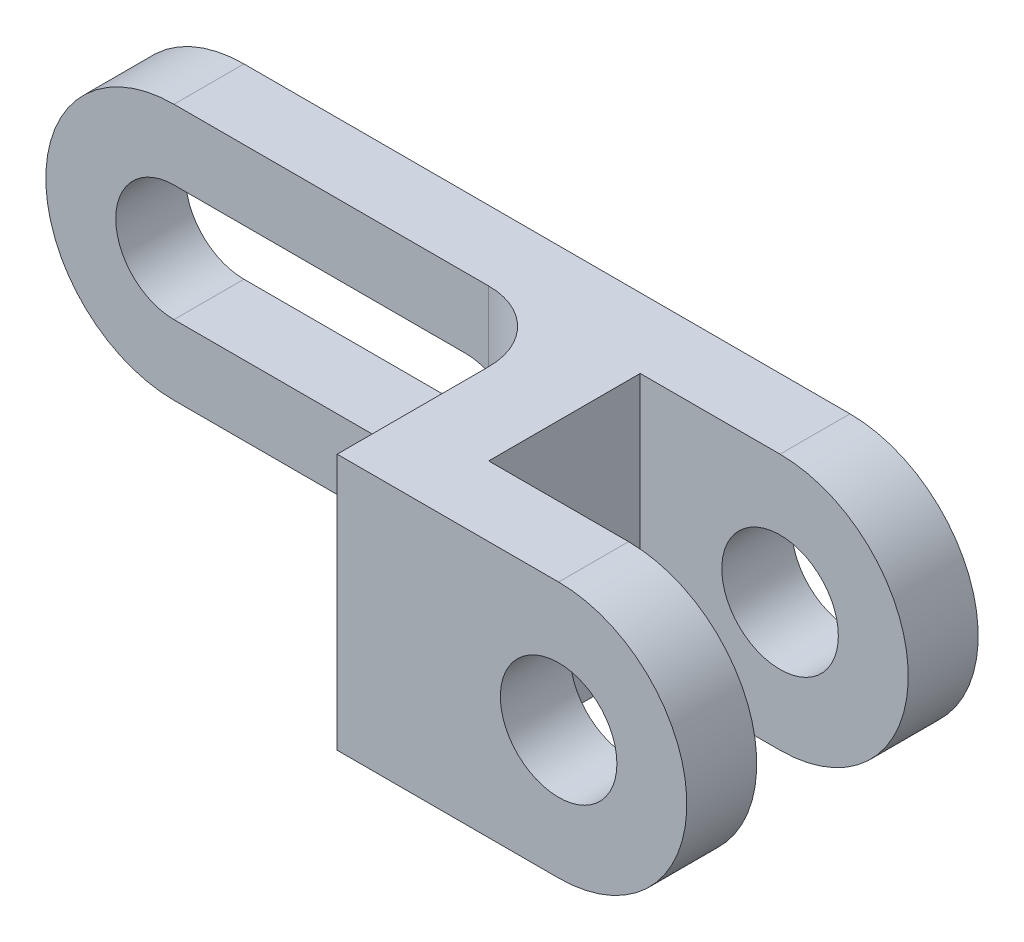
ISO-10303-21;
HEADER;
FILE_DESCRIPTION(('STEP AP214'),'2;1');
FILE_NAME('part.step','',(''),(''),'','','');
FILE_SCHEMA(('AUTOMOTIVE_DESIGN { 1 0 10303 214 1 1 1 1 }'));
ENDSEC;
DATA;
#1=APPLICATION_CONTEXT('core data for automotive mechanical design processes');
#2=APPLICATION_PROTOCOL_DEFINITION('international standard','automotive_design',2000,#1);
#3=PRODUCT_CONTEXT('',#1,'mechanical');
#4=PRODUCT('Part','Part','',(#3));
#5=PRODUCT_RELATED_PRODUCT_CATEGORY('part','',(#4));
#6=PRODUCT_DEFINITION_FORMATION('','',#4);
#7=PRODUCT_DEFINITION_CONTEXT('part definition',#1,'design');
#8=PRODUCT_DEFINITION('design','',#6,#7);
#9=PRODUCT_DEFINITION_SHAPE('','',#8);
#10=(LENGTH_UNIT() NAMED_UNIT(*) SI_UNIT(.MILLI.,.METRE.));
#11=(NAMED_UNIT(*) PLANE_ANGLE_UNIT() SI_UNIT($,.RADIAN.));
#12=(NAMED_UNIT(*) SI_UNIT($,.STERADIAN.) SOLID_ANGLE_UNIT());
#13=UNCERTAINTY_MEASURE_WITH_UNIT(LENGTH_MEASURE(1.E-05),#10,'distance_accuracy_value','');
#14=(GEOMETRIC_REPRESENTATION_CONTEXT(3) GLOBAL_UNCERTAINTY_ASSIGNED_CONTEXT((#13)) GLOBAL_UNIT_ASSIGNED_CONTEXT((#10,
#11,#12)) REPRESENTATION_CONTEXT('',''));
#15=CARTESIAN_POINT('',(0.,0.,0.));
#16=DIRECTION('',(0.,0.,1.));
#17=DIRECTION('',(1.,0.,0.));
#18=AXIS2_PLACEMENT_3D('',#15,#16,#17);
#19=CARTESIAN_POINT('',(0.,0.,6.));
#20=DIRECTION('',(0.,0.,1.));
#21=DIRECTION('',(1.,0.,0.));
#22=AXIS2_PLACEMENT_3D('',#19,#20,#21);
#23=PLANE('',#22);
#24=DIRECTION('',(1.,0.,0.));
#25=VECTOR('',#24,1.);
#26=CARTESIAN_POINT('',(52.,-11.,6.));
#27=LINE('',#26,#25);
#28=CARTESIAN_POINT('',(0.,-11.,6.));
#29=VERTEX_POINT('',#28);
#30=CARTESIAN_POINT('',(27.,-11.,6.));
#31=VERTEX_POINT('',#30);
#32=EDGE_CURVE('E260',#29,#31,#27,.T.);
#33=ORIENTED_EDGE('',*,*,#32,.T.);
#34=DIRECTION('',(0.,-1.,0.));
#35=VECTOR('',#34,1.);
#36=CARTESIAN_POINT('',(27.,11.,6.));
#37=LINE('',#36,#35);
#38=CARTESIAN_POINT('',(27.,-4.58257569495585,6.));
#39=VERTEX_POINT('',#38);
#40=EDGE_CURVE('E215',#39,#31,#37,.T.);
#41=ORIENTED_EDGE('',*,*,#40,.F.);
#42=CARTESIAN_POINT('',(25.,0.,6.));
#43=DIRECTION('',(0.,0.,1.));
#44=DIRECTION('',(1.,0.,0.));
#45=AXIS2_PLACEMENT_3D('',#42,#43,#44);
#46=CIRCLE('',#45,5.);
#47=CARTESIAN_POINT('',(25.,-5.,6.));
#48=VERTEX_POINT('',#47);
#49=EDGE_CURVE('E238',#48,#39,#46,.T.);
#50=ORIENTED_EDGE('',*,*,#49,.F.);
#51=DIRECTION('',(1.,0.,0.));
#52=VECTOR('',#51,1.);
#53=CARTESIAN_POINT('',(25.,-5.,6.));
#54=LINE('',#53,#52);
#55=CARTESIAN_POINT('',(0.,-5.,6.));
#56=VERTEX_POINT('',#55);
#57=EDGE_CURVE('E234',#56,#48,#54,.T.);
#58=ORIENTED_EDGE('',*,*,#57,.F.);
#59=CARTESIAN_POINT('',(0.,0.,6.));
#60=DIRECTION('',(0.,0.,1.));
#61=DIRECTION('',(1.,0.,0.));
#62=AXIS2_PLACEMENT_3D('',#59,#60,#61);
#63=CIRCLE('',#62,5.);
#64=CARTESIAN_POINT('',(0.,5.,6.));
#65=VERTEX_POINT('',#64);
#66=EDGE_CURVE('E62',#65,#56,#63,.T.);
#67=ORIENTED_EDGE('',*,*,#66,.F.);
#68=DIRECTION('',(-1.,0.,0.));
#69=VECTOR('',#68,1.);
#70=CARTESIAN_POINT('',(0.,5.,6.));
#71=LINE('',#70,#69);
#72=CARTESIAN_POINT('',(25.,5.,6.));
#73=VERTEX_POINT('',#72);
#74=EDGE_CURVE('E221',#73,#65,#71,.T.);
#75=ORIENTED_EDGE('',*,*,#74,.F.);
#76=CARTESIAN_POINT('',(27.,4.58257569495585,6.));
#77=VERTEX_POINT('',#76);
#78=EDGE_CURVE('E240',#77,#73,#46,.T.);
#79=ORIENTED_EDGE('',*,*,#78,.F.);
#80=CARTESIAN_POINT('',(27.,11.,6.));
#81=VERTEX_POINT('',#80);
#82=EDGE_CURVE('E209',#81,#77,#37,.T.);
#83=ORIENTED_EDGE('',*,*,#82,.F.);
#84=DIRECTION('',(-1.,0.,0.));
#85=VECTOR('',#84,1.);
#86=CARTESIAN_POINT('',(0.,11.,6.));
#87=LINE('',#86,#85);
#88=CARTESIAN_POINT('',(0.,11.,6.));
#89=VERTEX_POINT('',#88);
#90=EDGE_CURVE('E265',#81,#89,#87,.T.);
#91=ORIENTED_EDGE('',*,*,#90,.T.);
#92=CARTESIAN_POINT('',(0.,0.,6.));
#93=DIRECTION('',(0.,0.,1.));
#94=DIRECTION('',(1.,0.,0.));
#95=AXIS2_PLACEMENT_3D('',#92,#93,#94);
#96=CIRCLE('',#95,11.);
#97=EDGE_CURVE('E255',#89,#29,#96,.T.);
#98=ORIENTED_EDGE('',*,*,#97,.T.);
#99=EDGE_LOOP('',(#33,#41,#50,#58,#67,#75,#79,#83,#91,#98));
#100=FACE_BOUND('',#99,.T.);
#101=ADVANCED_FACE('F44',(#100),#23,.T.);
#102=CARTESIAN_POINT('',(0.,0.,6.));
#103=DIRECTION('',(0.,0.,-1.));
#104=DIRECTION('',(-1.,0.,0.));
#105=AXIS2_PLACEMENT_3D('',#102,#103,#104);
#106=CYLINDRICAL_SURFACE('',#105,11.);
#107=CARTESIAN_POINT('',(0.,0.,0.));
#108=DIRECTION('',(0.,0.,1.));
#109=DIRECTION('',(1.,0.,0.));
#110=AXIS2_PLACEMENT_3D('',#107,#108,#109);
#111=CIRCLE('',#110,11.);
#112=CARTESIAN_POINT('',(0.,11.,0.));
#113=VERTEX_POINT('',#112);
#114=CARTESIAN_POINT('',(0.,-11.,0.));
#115=VERTEX_POINT('',#114);
#116=EDGE_CURVE('E244',#113,#115,#111,.T.);
#117=ORIENTED_EDGE('',*,*,#116,.T.);
#118=DIRECTION('',(0.,0.,-1.));
#119=VECTOR('',#118,1.);
#120=CARTESIAN_POINT('',(0.,-11.,6.));
#121=LINE('',#120,#119);
#122=EDGE_CURVE('E53',#29,#115,#121,.T.);
#123=ORIENTED_EDGE('',*,*,#122,.F.);
#124=ORIENTED_EDGE('',*,*,#97,.F.);
#125=DIRECTION('',(0.,0.,-1.));
#126=VECTOR('',#125,1.);
#127=CARTESIAN_POINT('',(0.,11.,6.));
#128=LINE('',#127,#126);
#129=EDGE_CURVE('E267',#89,#113,#128,.T.);
#130=ORIENTED_EDGE('',*,*,#129,.T.);
#131=EDGE_LOOP('',(#117,#123,#124,#130));
#132=FACE_BOUND('',#131,.T.);
#133=ADVANCED_FACE('F50',(#132),#106,.T.);
#134=CARTESIAN_POINT('',(52.,-11.,6.));
#135=DIRECTION('',(0.,1.,0.));
#136=DIRECTION('',(0.,0.,1.));
#137=AXIS2_PLACEMENT_3D('',#134,#135,#136);
#138=PLANE('',#137);
#139=DIRECTION('',(1.,0.,0.));
#140=VECTOR('',#139,1.);
#141=CARTESIAN_POINT('',(52.,-11.,0.));
#142=LINE('',#141,#140);
#143=CARTESIAN_POINT('',(52.,-11.,0.));
#144=VERTEX_POINT('',#143);
#145=EDGE_CURVE('E269',#115,#144,#142,.T.);
#146=ORIENTED_EDGE('',*,*,#145,.T.);
#147=DIRECTION('',(0.,0.,-1.));
#148=VECTOR('',#147,1.);
#149=CARTESIAN_POINT('',(52.,-11.,6.));
#150=LINE('',#149,#148);
#151=CARTESIAN_POINT('',(52.,-11.,6.));
#152=VERTEX_POINT('',#151);
#153=EDGE_CURVE('E276',#152,#144,#150,.T.);
#154=ORIENTED_EDGE('',*,*,#153,.F.);
#155=CARTESIAN_POINT('',(40.,-11.,6.));
#156=VERTEX_POINT('',#155);
#157=EDGE_CURVE('E253',#156,#152,#27,.T.);
#158=ORIENTED_EDGE('',*,*,#157,.F.);
#159=DIRECTION('',(0.,0.,1.));
#160=VECTOR('',#159,1.);
#161=CARTESIAN_POINT('',(40.,-11.,6.));
#162=LINE('',#161,#160);
#163=CARTESIAN_POINT('',(40.,-11.,19.));
#164=VERTEX_POINT('',#163);
#165=EDGE_CURVE('E166',#156,#164,#162,.T.);
#166=ORIENTED_EDGE('',*,*,#165,.T.);
#167=DIRECTION('',(1.,0.,0.));
#168=VECTOR('',#167,1.);
#169=CARTESIAN_POINT('',(40.,-11.,19.));
#170=LINE('',#169,#168);
#171=CARTESIAN_POINT('',(52.,-11.,19.));
#172=VERTEX_POINT('',#171);
#173=EDGE_CURVE('E198',#164,#172,#170,.T.);
#174=ORIENTED_EDGE('',*,*,#173,.T.);
#175=DIRECTION('',(0.,0.,1.));
#176=VECTOR('',#175,1.);
#177=CARTESIAN_POINT('',(52.,-11.,25.));
#178=LINE('',#177,#176);
#179=CARTESIAN_POINT('',(52.,-11.,25.));
#180=VERTEX_POINT('',#179);
#181=EDGE_CURVE('E161',#172,#180,#178,.T.);
#182=ORIENTED_EDGE('',*,*,#181,.T.);
#183=DIRECTION('',(-1.,0.,0.));
#184=VECTOR('',#183,1.);
#185=CARTESIAN_POINT('',(33.,-11.,25.));
#186=LINE('',#185,#184);
#187=CARTESIAN_POINT('',(33.,-11.,25.));
#188=VERTEX_POINT('',#187);
#189=EDGE_CURVE('E202',#180,#188,#186,.T.);
#190=ORIENTED_EDGE('',*,*,#189,.T.);
#191=DIRECTION('',(0.,0.,-1.));
#192=VECTOR('',#191,1.);
#193=CARTESIAN_POINT('',(33.,-11.,12.));
#194=LINE('',#193,#192);
#195=CARTESIAN_POINT('',(33.,-11.,12.));
#196=VERTEX_POINT('',#195);
#197=EDGE_CURVE('E204',#188,#196,#194,.T.);
#198=ORIENTED_EDGE('',*,*,#197,.T.);
#199=CARTESIAN_POINT('',(27.,-11.,12.));
#200=DIRECTION('',(0.,1.,0.));
#201=DIRECTION('',(0.,0.,-1.));
#202=AXIS2_PLACEMENT_3D('',#199,#200,#201);
#203=CIRCLE('',#202,6.);
#204=EDGE_CURVE('E187',#196,#31,#203,.T.);
#205=ORIENTED_EDGE('',*,*,#204,.T.);
#206=ORIENTED_EDGE('',*,*,#32,.F.);
#207=ORIENTED_EDGE('',*,*,#122,.T.);
#208=EDGE_LOOP('',(#146,#154,#158,#166,#174,#182,#190,#198,#205,#206,#207));
#209=FACE_BOUND('',#208,.T.);
#210=ADVANCED_FACE('F320',(#209),#138,.F.);
#211=CARTESIAN_POINT('',(52.,0.,6.));
#212=DIRECTION('',(0.,0.,-1.));
#213=DIRECTION('',(-1.,0.,0.));
#214=AXIS2_PLACEMENT_3D('',#211,#212,#213);
#215=CYLINDRICAL_SURFACE('',#214,11.);
#216=CARTESIAN_POINT('',(52.,0.,0.));
#217=DIRECTION('',(0.,0.,1.));
#218=DIRECTION('',(1.,0.,0.));
#219=AXIS2_PLACEMENT_3D('',#216,#217,#218);
#220=CIRCLE('',#219,11.);
#221=CARTESIAN_POINT('',(52.,11.,0.));
#222=VERTEX_POINT('',#221);
#223=EDGE_CURVE('E272',#144,#222,#220,.T.);
#224=ORIENTED_EDGE('',*,*,#223,.T.);
#225=DIRECTION('',(0.,0.,-1.));
#226=VECTOR('',#225,1.);
#227=CARTESIAN_POINT('',(52.,11.,6.));
#228=LINE('',#227,#226);
#229=CARTESIAN_POINT('',(52.,11.,6.));
#230=VERTEX_POINT('',#229);
#231=EDGE_CURVE('E277',#230,#222,#228,.T.);
#232=ORIENTED_EDGE('',*,*,#231,.F.);
#233=CARTESIAN_POINT('',(52.,0.,6.));
#234=DIRECTION('',(0.,0.,1.));
#235=DIRECTION('',(1.,0.,0.));
#236=AXIS2_PLACEMENT_3D('',#233,#234,#235);
#237=CIRCLE('',#236,11.);
#238=EDGE_CURVE('E258',#152,#230,#237,.T.);
#239=ORIENTED_EDGE('',*,*,#238,.F.);
#240=ORIENTED_EDGE('',*,*,#153,.T.);
#241=EDGE_LOOP('',(#224,#232,#239,#240));
#242=FACE_BOUND('',#241,.T.);
#243=ADVANCED_FACE('F332',(#242),#215,.T.);
#244=CARTESIAN_POINT('',(0.,11.,6.));
#245=DIRECTION('',(0.,-1.,0.));
#246=DIRECTION('',(0.,0.,-1.));
#247=AXIS2_PLACEMENT_3D('',#244,#245,#246);
#248=PLANE('',#247);
#249=DIRECTION('',(-1.,0.,0.));
#250=VECTOR('',#249,1.);
#251=CARTESIAN_POINT('',(0.,11.,0.));
#252=LINE('',#251,#250);
#253=EDGE_CURVE('E257',#222,#113,#252,.T.);
#254=ORIENTED_EDGE('',*,*,#253,.T.);
#255=ORIENTED_EDGE('',*,*,#129,.F.);
#256=ORIENTED_EDGE('',*,*,#90,.F.);
#257=CARTESIAN_POINT('',(27.,11.,12.));
#258=DIRECTION('',(0.,1.,0.));
#259=DIRECTION('',(0.,0.,-1.));
#260=AXIS2_PLACEMENT_3D('',#257,#258,#259);
#261=CIRCLE('',#260,6.);
#262=CARTESIAN_POINT('',(33.,11.,12.));
#263=VERTEX_POINT('',#262);
#264=EDGE_CURVE('E194',#263,#81,#261,.T.);
#265=ORIENTED_EDGE('',*,*,#264,.F.);
#266=DIRECTION('',(0.,0.,-1.));
#267=VECTOR('',#266,1.);
#268=CARTESIAN_POINT('',(33.,11.,19.));
#269=LINE('',#268,#267);
#270=CARTESIAN_POINT('',(33.,11.,25.));
#271=VERTEX_POINT('',#270);
#272=EDGE_CURVE('E192',#271,#263,#269,.T.);
#273=ORIENTED_EDGE('',*,*,#272,.F.);
#274=DIRECTION('',(-1.,0.,0.));
#275=VECTOR('',#274,1.);
#276=CARTESIAN_POINT('',(33.,11.,25.));
#277=LINE('',#276,#275);
#278=CARTESIAN_POINT('',(52.,11.,25.));
#279=VERTEX_POINT('',#278);
#280=EDGE_CURVE('E179',#279,#271,#277,.T.);
#281=ORIENTED_EDGE('',*,*,#280,.F.);
#282=DIRECTION('',(0.,0.,1.));
#283=VECTOR('',#282,1.);
#284=CARTESIAN_POINT('',(52.,11.,25.));
#285=LINE('',#284,#283);
#286=CARTESIAN_POINT('',(52.,11.,19.));
#287=VERTEX_POINT('',#286);
#288=EDGE_CURVE('E156',#287,#279,#285,.T.);
#289=ORIENTED_EDGE('',*,*,#288,.F.);
#290=DIRECTION('',(1.,0.,0.));
#291=VECTOR('',#290,1.);
#292=CARTESIAN_POINT('',(40.,11.,19.));
#293=LINE('',#292,#291);
#294=CARTESIAN_POINT('',(40.,11.,19.));
#295=VERTEX_POINT('',#294);
#296=EDGE_CURVE('E176',#295,#287,#293,.T.);
#297=ORIENTED_EDGE('',*,*,#296,.F.);
#298=DIRECTION('',(0.,0.,1.));
#299=VECTOR('',#298,1.);
#300=CARTESIAN_POINT('',(40.,11.,6.));
#301=LINE('',#300,#299);
#302=CARTESIAN_POINT('',(40.,11.,6.));
#303=VERTEX_POINT('',#302);
#304=EDGE_CURVE('E183',#303,#295,#301,.T.);
#305=ORIENTED_EDGE('',*,*,#304,.F.);
#306=EDGE_CURVE('E263',#230,#303,#87,.T.);
#307=ORIENTED_EDGE('',*,*,#306,.F.);
#308=ORIENTED_EDGE('',*,*,#231,.T.);
#309=EDGE_LOOP('',(#254,#255,#256,#265,#273,#281,#289,#297,#305,#307,#308));
#310=FACE_BOUND('',#309,.T.);
#311=ADVANCED_FACE('F172',(#310),#248,.F.);
#312=CARTESIAN_POINT('',(52.,0.,6.));
#313=DIRECTION('',(0.,0.,1.));
#314=DIRECTION('',(1.,0.,0.));
#315=AXIS2_PLACEMENT_3D('',#312,#313,#314);
#316=CIRCLE('',#315,5.);
#317=CARTESIAN_POINT('',(57.,0.,6.));
#318=VERTEX_POINT('',#317);
#319=EDGE_CURVE('E337',#318,#318,#316,.T.);
#320=ORIENTED_EDGE('',*,*,#319,.F.);
#321=EDGE_LOOP('',(#320));
#322=FACE_BOUND('',#321,.T.);
#323=DIRECTION('',(0.,-1.,0.));
#324=VECTOR('',#323,1.);
#325=CARTESIAN_POINT('',(40.,11.,6.));
#326=LINE('',#325,#324);
#327=EDGE_CURVE('E193',#303,#156,#326,.T.);
#328=ORIENTED_EDGE('',*,*,#327,.T.);
#329=ORIENTED_EDGE('',*,*,#157,.T.);
#330=ORIENTED_EDGE('',*,*,#238,.T.);
#331=ORIENTED_EDGE('',*,*,#306,.T.);
#332=EDGE_LOOP('',(#328,#329,#330,#331));
#333=FACE_BOUND('',#332,.T.);
#334=ADVANCED_FACE('F311',(#322,#333),#23,.T.);
#335=CARTESIAN_POINT('',(0.,0.,0.));
#336=DIRECTION('',(0.,0.,1.));
#337=DIRECTION('',(1.,0.,0.));
#338=AXIS2_PLACEMENT_3D('',#335,#336,#337);
#339=PLANE('',#338);
#340=CARTESIAN_POINT('',(52.,0.,0.));
#341=DIRECTION('',(0.,0.,1.));
#342=DIRECTION('',(1.,0.,0.));
#343=AXIS2_PLACEMENT_3D('',#340,#341,#342);
#344=CIRCLE('',#343,5.);
#345=CARTESIAN_POINT('',(57.,0.,0.));
#346=VERTEX_POINT('',#345);
#347=EDGE_CURVE('E597',#346,#346,#344,.T.);
#348=ORIENTED_EDGE('',*,*,#347,.T.);
#349=EDGE_LOOP('',(#348));
#350=FACE_BOUND('',#349,.T.);
#351=DIRECTION('',(-1.,0.,0.));
#352=VECTOR('',#351,1.);
#353=CARTESIAN_POINT('',(0.,5.,0.));
#354=LINE('',#353,#352);
#355=CARTESIAN_POINT('',(25.,5.,0.));
#356=VERTEX_POINT('',#355);
#357=CARTESIAN_POINT('',(0.,5.,0.));
#358=VERTEX_POINT('',#357);
#359=EDGE_CURVE('E230',#356,#358,#354,.T.);
#360=ORIENTED_EDGE('',*,*,#359,.T.);
#361=CARTESIAN_POINT('',(0.,0.,0.));
#362=DIRECTION('',(0.,0.,1.));
#363=DIRECTION('',(1.,0.,0.));
#364=AXIS2_PLACEMENT_3D('',#361,#362,#363);
#365=CIRCLE('',#364,5.);
#366=CARTESIAN_POINT('',(0.,-5.,0.));
#367=VERTEX_POINT('',#366);
#368=EDGE_CURVE('E222',#358,#367,#365,.T.);
#369=ORIENTED_EDGE('',*,*,#368,.T.);
#370=DIRECTION('',(1.,0.,0.));
#371=VECTOR('',#370,1.);
#372=CARTESIAN_POINT('',(25.,-5.,0.));
#373=LINE('',#372,#371);
#374=CARTESIAN_POINT('',(25.,-5.,0.));
#375=VERTEX_POINT('',#374);
#376=EDGE_CURVE('E224',#367,#375,#373,.T.);
#377=ORIENTED_EDGE('',*,*,#376,.T.);
#378=CARTESIAN_POINT('',(25.,0.,0.));
#379=DIRECTION('',(0.,0.,1.));
#380=DIRECTION('',(1.,0.,0.));
#381=AXIS2_PLACEMENT_3D('',#378,#379,#380);
#382=CIRCLE('',#381,5.);
#383=EDGE_CURVE('E67',#375,#356,#382,.T.);
#384=ORIENTED_EDGE('',*,*,#383,.T.);
#385=EDGE_LOOP('',(#360,#369,#377,#384));
#386=FACE_BOUND('',#385,.T.);
#387=ORIENTED_EDGE('',*,*,#116,.F.);
#388=ORIENTED_EDGE('',*,*,#253,.F.);
#389=ORIENTED_EDGE('',*,*,#223,.F.);
#390=ORIENTED_EDGE('',*,*,#145,.F.);
#391=EDGE_LOOP('',(#387,#388,#389,#390));
#392=FACE_BOUND('',#391,.T.);
#393=ADVANCED_FACE('F325',(#350,#386,#392),#339,.F.);
#394=CARTESIAN_POINT('',(0.,0.,0.));
#395=DIRECTION('',(0.,0.,1.));
#396=DIRECTION('',(1.,0.,0.));
#397=AXIS2_PLACEMENT_3D('',#394,#395,#396);
#398=CYLINDRICAL_SURFACE('',#397,5.);
#399=ORIENTED_EDGE('',*,*,#66,.T.);
#400=DIRECTION('',(0.,0.,1.));
#401=VECTOR('',#400,1.);
#402=CARTESIAN_POINT('',(0.,-5.,0.));
#403=LINE('',#402,#401);
#404=EDGE_CURVE('E235',#367,#56,#403,.T.);
#405=ORIENTED_EDGE('',*,*,#404,.F.);
#406=ORIENTED_EDGE('',*,*,#368,.F.);
#407=DIRECTION('',(0.,0.,1.));
#408=VECTOR('',#407,1.);
#409=CARTESIAN_POINT('',(0.,5.,0.));
#410=LINE('',#409,#408);
#411=EDGE_CURVE('E243',#358,#65,#410,.T.);
#412=ORIENTED_EDGE('',*,*,#411,.T.);
#413=EDGE_LOOP('',(#399,#405,#406,#412));
#414=FACE_BOUND('',#413,.T.);
#415=ADVANCED_FACE('F328',(#414),#398,.F.);
#416=CARTESIAN_POINT('',(0.,5.,0.));
#417=DIRECTION('',(0.,1.,0.));
#418=DIRECTION('',(-1.,0.,0.));
#419=AXIS2_PLACEMENT_3D('',#416,#417,#418);
#420=PLANE('',#419);
#421=ORIENTED_EDGE('',*,*,#74,.T.);
#422=ORIENTED_EDGE('',*,*,#411,.F.);
#423=ORIENTED_EDGE('',*,*,#359,.F.);
#424=DIRECTION('',(0.,0.,1.));
#425=VECTOR('',#424,1.);
#426=CARTESIAN_POINT('',(25.,5.,0.));
#427=LINE('',#426,#425);
#428=EDGE_CURVE('E246',#356,#73,#427,.T.);
#429=ORIENTED_EDGE('',*,*,#428,.T.);
#430=EDGE_LOOP('',(#421,#422,#423,#429));
#431=FACE_BOUND('',#430,.T.);
#432=ADVANCED_FACE('F364',(#431),#420,.F.);
#433=CARTESIAN_POINT('',(25.,0.,0.));
#434=DIRECTION('',(0.,0.,1.));
#435=DIRECTION('',(1.,0.,0.));
#436=AXIS2_PLACEMENT_3D('',#433,#434,#435);
#437=CYLINDRICAL_SURFACE('',#436,5.);
#438=ORIENTED_EDGE('',*,*,#49,.T.);
#439=CARTESIAN_POINT('',(27.,-4.58257569495585,6.));
#440=CARTESIAN_POINT('',(27.1217437345548,-4.5294693831626,5.9999795322842));
#441=CARTESIAN_POINT('',(27.2412946033694,-4.47149264236447,6.00370425354419));
#442=CARTESIAN_POINT('',(27.4750029468276,-4.34647410640989,6.01769324070108));
#443=CARTESIAN_POINT('',(27.5891661032485,-4.27944216261416,6.0279504441919));
#444=CARTESIAN_POINT('',(27.8106587466322,-4.13732040188335,6.053975439873));
#445=CARTESIAN_POINT('',(27.9180267204908,-4.06228395381264,6.06970814387246));
#446=CARTESIAN_POINT('',(28.1260824180399,-3.90444340002841,6.10567271479802));
#447=CARTESIAN_POINT('',(28.2267684172859,-3.82163730237625,6.12590573732239));
#448=CARTESIAN_POINT('',(28.5172296080022,-3.56314405726873,6.19162235963019));
#449=CARTESIAN_POINT('',(28.6964613733419,-3.37670120504686,6.24226566813938));
#450=CARTESIAN_POINT('',(29.0237888926283,-2.97922021325291,6.34897723583559));
#451=CARTESIAN_POINT('',(29.1718123574958,-2.7681266927584,6.40505766033279));
#452=CARTESIAN_POINT('',(29.4470649308166,-2.30292442140226,6.51946610020983));
#453=CARTESIAN_POINT('',(29.5708014386373,-2.04662652366791,6.57746995237268));
#454=CARTESIAN_POINT('',(29.7228694474649,-1.6476695672957,6.65311571588317));
#455=CARTESIAN_POINT('',(29.7679700276443,-1.51226202487204,6.67643807219076));
#456=CARTESIAN_POINT('',(29.8465708518994,-1.23739317483382,6.71804776237524));
#457=CARTESIAN_POINT('',(29.8800777617572,-1.09793424673085,6.73633798823267));
#458=CARTESIAN_POINT('',(29.933999372941,-0.821419761269932,6.76620954045993));
#459=CARTESIAN_POINT('',(29.9548672276227,-0.684477413321925,6.77802142801882));
#460=CARTESIAN_POINT('',(29.9851762466153,-0.408928152222863,6.79528765245774));
#461=CARTESIAN_POINT('',(29.9946178087185,-0.270321297189237,6.80074221066007));
#462=CARTESIAN_POINT('',(30.0019210038343,0.00723999453303636,6.80495539479658));
#463=CARTESIAN_POINT('',(29.9997875826259,0.146194257416662,6.80371688055934));
#464=CARTESIAN_POINT('',(29.9839877306749,0.423218153370086,6.79462781772828));
#465=CARTESIAN_POINT('',(29.9703219511779,0.561287835949559,6.78677764250277));
#466=CARTESIAN_POINT('',(29.9338737060189,0.819710467078495,6.76619016242889));
#467=CARTESIAN_POINT('',(29.9123071211526,0.940289918625227,6.75411145344576));
#468=CARTESIAN_POINT('',(29.8605260577144,1.17908066461603,6.72569857253865));
#469=CARTESIAN_POINT('',(29.8303087393953,1.29729116775655,6.70936300338774));
#470=CARTESIAN_POINT('',(29.727082374066,1.64736215701917,6.65499096497028));
#471=CARTESIAN_POINT('',(29.6414798754925,1.87479473181708,6.61157732218962));
#472=CARTESIAN_POINT('',(29.4312208674812,2.3307357050401,6.51332375558086));
#473=CARTESIAN_POINT('',(29.304018434822,2.55791663482714,6.45785301328951));
#474=CARTESIAN_POINT('',(29.0157370062914,2.99020640278438,6.34662498799436));
#475=CARTESIAN_POINT('',(28.8546139801217,3.19528602429615,6.29086742536242));
#476=CARTESIAN_POINT('',(28.5803844459976,3.49308678962271,6.21098012277737));
#477=CARTESIAN_POINT('',(28.4780105233846,3.59505383825582,6.18385401462426));
#478=CARTESIAN_POINT('',(28.2642800189335,3.79016912849186,6.13368722879749));
#479=CARTESIAN_POINT('',(28.1529277823403,3.88332158921457,6.11064459190513));
#480=CARTESIAN_POINT('',(27.9222342107592,4.05975129785079,6.07014634878593));
#481=CARTESIAN_POINT('',(27.8029173103952,4.1430567566569,6.05267452583132));
#482=CARTESIAN_POINT('',(27.5569483230002,4.29920836926142,6.02462588412011));
#483=CARTESIAN_POINT('',(27.4303033751533,4.37206447011965,6.01404247365259));
#484=CARTESIAN_POINT('',(27.2513254517487,4.4648203876681,6.00506246920854));
#485=CARTESIAN_POINT('',(27.2016104335286,4.48954311990866,6.00317841469992));
#486=CARTESIAN_POINT('',(27.101389688586,4.53731624274857,6.00064757298348));
#487=CARTESIAN_POINT('',(27.0508844614831,4.56036764194023,6.00000003350095));
#488=CARTESIAN_POINT('',(27.,4.58257569495585,6.));
#489=B_SPLINE_CURVE_WITH_KNOTS('',3,(#439,#440,#441,#442,#443,#444,#445,#446,#447,#448,#449,
#450,#451,#452,#453,#454,#455,#456,#457,#458,#459,#460,#461,#462,#463,#464,#465,#466,#467,#468,
#469,#470,#471,#472,#473,#474,#475,#476,#477,#478,#479,#480,#481,#482,#483,#484,#485,#486,#487,
#488),.UNSPECIFIED.,.F.,.F.,(4,2,2,2,2,2,2,2,2,2,2,2,2,2,2,2,2,2,2,2,2,2,2,2,4),(0.,
0.398216398207483,0.796003005308236,1.19128606960233,1.58667075267249,2.37369907727779,
3.16253087157769,4.0291919544517,4.46254399445514,4.89564646301965,5.31212518720737,
5.72858941178641,6.14487570282172,6.56113848725511,6.92998209195776,7.29894691482475,
8.03647761473628,8.83212604378076,9.6288136956455,10.0693642279109,10.5097028116827,
10.9487476054058,11.3873716450054,11.5540007401415,11.720528428632),.UNSPECIFIED.);
#490=EDGE_CURVE('E11',#39,#77,#489,.T.);
#491=ORIENTED_EDGE('',*,*,#490,.T.);
#492=ORIENTED_EDGE('',*,*,#78,.T.);
#493=ORIENTED_EDGE('',*,*,#428,.F.);
#494=ORIENTED_EDGE('',*,*,#383,.F.);
#495=DIRECTION('',(0.,0.,1.));
#496=VECTOR('',#495,1.);
#497=CARTESIAN_POINT('',(25.,-5.,0.));
#498=LINE('',#497,#496);
#499=EDGE_CURVE('E248',#375,#48,#498,.T.);
#500=ORIENTED_EDGE('',*,*,#499,.T.);
#501=EDGE_LOOP('',(#438,#491,#492,#493,#494,#500));
#502=FACE_BOUND('',#501,.T.);
#503=ADVANCED_FACE('F363',(#502),#437,.F.);
#504=CARTESIAN_POINT('',(25.,-5.,0.));
#505=DIRECTION('',(0.,-1.,0.));
#506=DIRECTION('',(1.,0.,0.));
#507=AXIS2_PLACEMENT_3D('',#504,#505,#506);
#508=PLANE('',#507);
#509=ORIENTED_EDGE('',*,*,#57,.T.);
#510=ORIENTED_EDGE('',*,*,#499,.F.);
#511=ORIENTED_EDGE('',*,*,#376,.F.);
#512=ORIENTED_EDGE('',*,*,#404,.T.);
#513=EDGE_LOOP('',(#509,#510,#511,#512));
#514=FACE_BOUND('',#513,.T.);
#515=ADVANCED_FACE('F369',(#514),#508,.F.);
#516=CARTESIAN_POINT('',(27.,11.,12.));
#517=DIRECTION('',(0.,-1.,0.));
#518=DIRECTION('',(0.,0.,-1.));
#519=AXIS2_PLACEMENT_3D('',#516,#517,#518);
#520=CYLINDRICAL_SURFACE('',#519,6.);
#521=ORIENTED_EDGE('',*,*,#490,.F.);
#522=ORIENTED_EDGE('',*,*,#40,.T.);
#523=ORIENTED_EDGE('',*,*,#204,.F.);
#524=DIRECTION('',(0.,-1.,0.));
#525=VECTOR('',#524,1.);
#526=CARTESIAN_POINT('',(33.,11.,12.));
#527=LINE('',#526,#525);
#528=EDGE_CURVE('E214',#263,#196,#527,.T.);
#529=ORIENTED_EDGE('',*,*,#528,.F.);
#530=ORIENTED_EDGE('',*,*,#264,.T.);
#531=ORIENTED_EDGE('',*,*,#82,.T.);
#532=EDGE_LOOP('',(#521,#522,#523,#529,#530,#531));
#533=FACE_BOUND('',#532,.T.);
#534=ADVANCED_FACE('F289',(#533),#520,.F.);
#535=CARTESIAN_POINT('',(33.,11.,12.));
#536=DIRECTION('',(-1.,0.,0.));
#537=DIRECTION('',(0.,0.,1.));
#538=AXIS2_PLACEMENT_3D('',#535,#536,#537);
#539=PLANE('',#538);
#540=ORIENTED_EDGE('',*,*,#197,.F.);
#541=DIRECTION('',(0.,-1.,0.));
#542=VECTOR('',#541,1.);
#543=CARTESIAN_POINT('',(33.,11.,25.));
#544=LINE('',#543,#542);
#545=EDGE_CURVE('E213',#271,#188,#544,.T.);
#546=ORIENTED_EDGE('',*,*,#545,.F.);
#547=ORIENTED_EDGE('',*,*,#272,.T.);
#548=ORIENTED_EDGE('',*,*,#528,.T.);
#549=EDGE_LOOP('',(#540,#546,#547,#548));
#550=FACE_BOUND('',#549,.T.);
#551=ADVANCED_FACE('F352',(#550),#539,.T.);
#552=CARTESIAN_POINT('',(33.,11.,25.));
#553=DIRECTION('',(0.,0.,1.));
#554=DIRECTION('',(1.,0.,0.));
#555=AXIS2_PLACEMENT_3D('',#552,#553,#554);
#556=PLANE('',#555);
#557=CARTESIAN_POINT('',(52.,0.,25.));
#558=DIRECTION('',(0.,0.,1.));
#559=DIRECTION('',(1.,0.,0.));
#560=AXIS2_PLACEMENT_3D('',#557,#558,#559);
#561=CIRCLE('',#560,5.);
#562=CARTESIAN_POINT('',(57.,0.,25.));
#563=VERTEX_POINT('',#562);
#564=EDGE_CURVE('E591',#563,#563,#561,.T.);
#565=ORIENTED_EDGE('',*,*,#564,.F.);
#566=EDGE_LOOP('',(#565));
#567=FACE_BOUND('',#566,.T.);
#568=ORIENTED_EDGE('',*,*,#189,.F.);
#569=CARTESIAN_POINT('',(52.,0.,25.));
#570=DIRECTION('',(0.,0.,1.));
#571=DIRECTION('',(1.,0.,0.));
#572=AXIS2_PLACEMENT_3D('',#569,#570,#571);
#573=CIRCLE('',#572,11.);
#574=EDGE_CURVE('E169',#180,#279,#573,.T.);
#575=ORIENTED_EDGE('',*,*,#574,.T.);
#576=ORIENTED_EDGE('',*,*,#280,.T.);
#577=ORIENTED_EDGE('',*,*,#545,.T.);
#578=EDGE_LOOP('',(#568,#575,#576,#577));
#579=FACE_BOUND('',#578,.T.);
#580=ADVANCED_FACE('F347',(#567,#579),#556,.T.);
#581=CARTESIAN_POINT('',(40.,11.,19.));
#582=DIRECTION('',(0.,0.,-1.));
#583=DIRECTION('',(-1.,0.,0.));
#584=AXIS2_PLACEMENT_3D('',#581,#582,#583);
#585=PLANE('',#584);
#586=CARTESIAN_POINT('',(52.,0.,19.));
#587=DIRECTION('',(0.,0.,-1.));
#588=DIRECTION('',(-1.,0.,0.));
#589=AXIS2_PLACEMENT_3D('',#586,#587,#588);
#590=CIRCLE('',#589,5.);
#591=CARTESIAN_POINT('',(47.,0.,19.));
#592=VERTEX_POINT('',#591);
#593=EDGE_CURVE('E47',#592,#592,#590,.T.);
#594=ORIENTED_EDGE('',*,*,#593,.F.);
#595=EDGE_LOOP('',(#594));
#596=FACE_BOUND('',#595,.T.);
#597=ORIENTED_EDGE('',*,*,#173,.F.);
#598=DIRECTION('',(0.,-1.,0.));
#599=VECTOR('',#598,1.);
#600=CARTESIAN_POINT('',(40.,11.,19.));
#601=LINE('',#600,#599);
#602=EDGE_CURVE('E182',#295,#164,#601,.T.);
#603=ORIENTED_EDGE('',*,*,#602,.F.);
#604=ORIENTED_EDGE('',*,*,#296,.T.);
#605=CARTESIAN_POINT('',(52.,0.,19.));
#606=DIRECTION('',(0.,0.,1.));
#607=DIRECTION('',(1.,0.,0.));
#608=AXIS2_PLACEMENT_3D('',#605,#606,#607);
#609=CIRCLE('',#608,11.);
#610=EDGE_CURVE('E160',#172,#287,#609,.T.);
#611=ORIENTED_EDGE('',*,*,#610,.F.);
#612=EDGE_LOOP('',(#597,#603,#604,#611));
#613=FACE_BOUND('',#612,.T.);
#614=ADVANCED_FACE('F185',(#596,#613),#585,.T.);
#615=CARTESIAN_POINT('',(40.,11.,6.));
#616=DIRECTION('',(1.,0.,0.));
#617=DIRECTION('',(0.,0.,-1.));
#618=AXIS2_PLACEMENT_3D('',#615,#616,#617);
#619=PLANE('',#618);
#620=ORIENTED_EDGE('',*,*,#165,.F.);
#621=ORIENTED_EDGE('',*,*,#327,.F.);
#622=ORIENTED_EDGE('',*,*,#304,.T.);
#623=ORIENTED_EDGE('',*,*,#602,.T.);
#624=EDGE_LOOP('',(#620,#621,#622,#623));
#625=FACE_BOUND('',#624,.T.);
#626=ADVANCED_FACE('F300',(#625),#619,.T.);
#627=CARTESIAN_POINT('',(52.,0.,19.));
#628=DIRECTION('',(0.,0.,1.));
#629=DIRECTION('',(1.,0.,0.));
#630=AXIS2_PLACEMENT_3D('',#627,#628,#629);
#631=CYLINDRICAL_SURFACE('',#630,11.);
#632=ORIENTED_EDGE('',*,*,#574,.F.);
#633=ORIENTED_EDGE('',*,*,#181,.F.);
#634=ORIENTED_EDGE('',*,*,#610,.T.);
#635=ORIENTED_EDGE('',*,*,#288,.T.);
#636=EDGE_LOOP('',(#632,#633,#634,#635));
#637=FACE_BOUND('',#636,.T.);
#638=ADVANCED_FACE('F159',(#637),#631,.T.);
#639=CARTESIAN_POINT('',(52.,0.,0.));
#640=DIRECTION('',(0.,0.,1.));
#641=DIRECTION('',(1.,0.,0.));
#642=AXIS2_PLACEMENT_3D('',#639,#640,#641);
#643=CYLINDRICAL_SURFACE('',#642,5.);
#644=ORIENTED_EDGE('',*,*,#593,.T.);
#645=EDGE_LOOP('',(#644));
#646=FACE_BOUND('',#645,.T.);
#647=ORIENTED_EDGE('',*,*,#564,.T.);
#648=EDGE_LOOP('',(#647));
#649=FACE_BOUND('',#648,.T.);
#650=ADVANCED_FACE('F298',(#646,#649),#643,.F.);
#651=ORIENTED_EDGE('',*,*,#319,.T.);
#652=EDGE_LOOP('',(#651));
#653=FACE_BOUND('',#652,.T.);
#654=ORIENTED_EDGE('',*,*,#347,.F.);
#655=EDGE_LOOP('',(#654));
#656=FACE_BOUND('',#655,.T.);
#657=ADVANCED_FACE('F299',(#653,#656),#643,.F.);
#658=CLOSED_SHELL('',(#101,#133,#210,#243,#311,#334,#393,#415,#432,#503,#515,#534,#551,#580,
#614,#626,#638,#650,#657));
#659=MANIFOLD_SOLID_BREP('B2',#658);
#660=ADVANCED_BREP_SHAPE_REPRESENTATION('',(#18,#659),#14);
#661=SHAPE_DEFINITION_REPRESENTATION(#9,#660);
ENDSEC;
END-ISO-10303-21;
